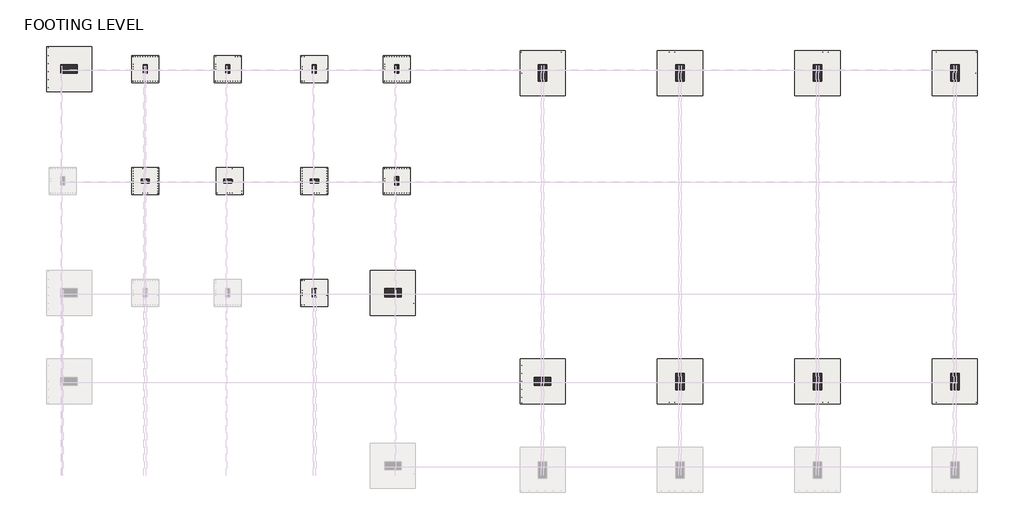
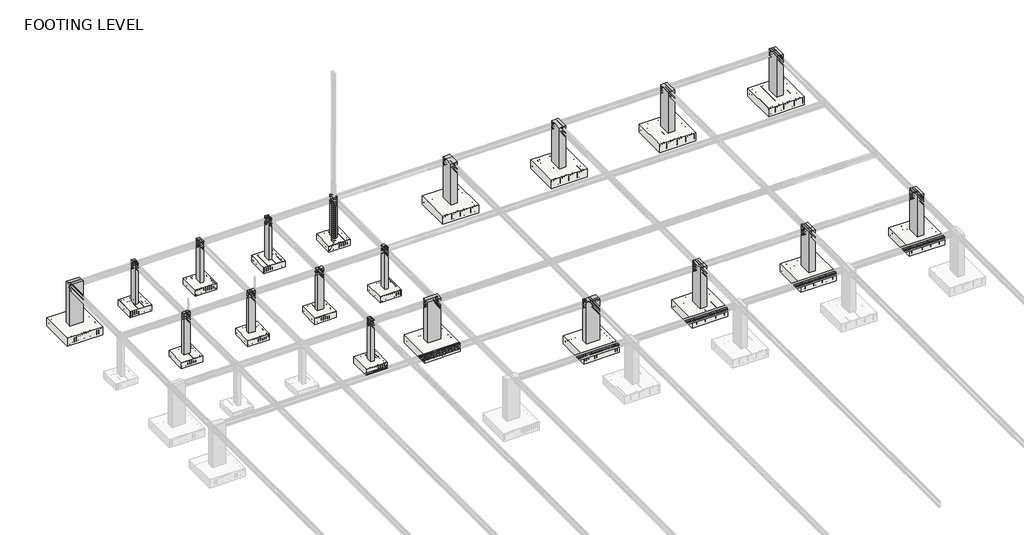
# One storey, part 2 of 19: 19 columns, 19 slabs.
"""IFC4 building model written with IfcOpenShell, lengths in millimetres."""

from ifc_helpers import new_model, si_unit, frame, origin, place, context, project, spatial, polyline, outline, extrude, faceted_brep, transform, mapped, element, save
from components import m_footing_rectangular_2500_x_2500_x_600_5d9c2050

model = new_model("IFC4")

# Units and contexts
model_context = context("Model", 3, world=origin())
ifc_project = project(units=[si_unit("LENGTHUNIT", "METRE", prefix="MILLI")], contexts=[model_context])

# Site, building, storey
site = spatial("IfcSite", under=ifc_project)
building = spatial("IfcBuilding", under=site)
storey = spatial("IfcBuildingStorey", under=building, Name="FOOTING LEVEL", Elevation=-3048.0)

# Columns
placement = place(None, origin())
element("IfcColumn", 1, ObjectType="M_Concrete-Rectangular-Column : 18\" X 36\"", at=placement, inside=storey, context=model_context, shape_type="Brep", body=[
    faceted_brep([(689.5587563, 6154.1794445, -3048.0), (1603.9587563, 6154.1794445, -3048.0), (1603.9587563, 5696.9794445, -3048.0), (689.5587563, 5696.9794445, -3048.0), (689.5587563, 6154.1794445, 0.0), (1603.9587563, 6154.1794445, 0.0), (1603.9587563, 5696.9794445, 0.0), (689.5587563, 5696.9794445, 0.0), (689.5587563, 5811.2794445, 0.0), (689.5587563, 6039.8794445, 0.0)], [[[0, 1, 2, 3]], [[4, 5, 1, 0]], [[5, 6, 2, 1]], [[6, 7, 3, 2]], [[7, 8, 9, 4, 0, 3]], [[4, 9, 8, 7, 6, 5]]]),
])
element("IfcColumn", 2, ObjectType="M_Concrete-Rectangular-Column : 18\" X 36\"", at=placement, inside=storey, context=model_context, shape_type="Brep", body=[
    faceted_brep([(32083.9587563, 553.4794445, -3048.0), (32083.9587563, 1467.8794445, -3048.0), (32541.1587563, 1467.8794445, -3048.0), (32541.1587563, 553.4794445, -3048.0), (32083.9587563, 553.4794445, 0.0), (32083.9587563, 1467.8794445, 0.0), (32198.2587563, 1467.8794445, 0.0), (32426.8587563, 1467.8794445, 0.0), (32541.1587563, 1467.8794445, 0.0), (32541.1587563, 553.4794445, 0.0), (32426.8587563, 553.4794445, 0.0), (32198.2587563, 553.4794445, 0.0)], [[[0, 1, 2, 3]], [[4, 5, 1, 0]], [[5, 6, 7, 8, 2, 1]], [[8, 9, 3, 2]], [[9, 10, 11, 4, 0, 3]], [[4, 11, 10, 9, 8, 7, 6, 5]]]),
])
element("IfcColumn", 3, ObjectType="M_Concrete-Rectangular-Column : 18\" X 36\"", at=placement, inside=storey, context=model_context, shape_type="Brep", body=[
    faceted_brep([(24463.9587563, 553.4794445, -3048.0), (24463.9587563, 1467.8794445, -3048.0), (24921.1587563, 1467.8794445, -3048.0), (24921.1587563, 553.4794445, -3048.0), (24463.9587563, 553.4794445, 0.0), (24463.9587563, 896.3794445, 0.0), (24463.9587563, 1124.9794445, 0.0), (24463.9587563, 1467.8794445, 0.0), (24578.2587563, 1467.8794445, 0.0), (24806.8587563, 1467.8794445, 0.0), (24921.1587563, 1467.8794445, 0.0), (24921.1587563, 1124.9794445, 0.0), (24921.1587563, 896.3794445, 0.0), (24921.1587563, 553.4794445, 0.0), (24806.8587563, 553.4794445, 0.0), (24578.2587563, 553.4794445, 0.0)], [[[0, 1, 2, 3]], [[4, 5, 6, 7, 1, 0]], [[7, 8, 9, 10, 2, 1]], [[10, 11, 12, 13, 3, 2]], [[13, 14, 15, 4, 0, 3]], [[4, 15, 14, 13, 12, 11, 10, 9, 8, 7, 6, 5]]]),
])
element("IfcColumn", 4, ObjectType="M_Concrete-Rectangular-Column : 18\" X 36\"", at=placement, inside=storey, context=model_context, shape_type="Brep", body=[
    faceted_brep([(16843.9587563, 553.4794445, -3048.0), (16843.9587563, 1467.8794445, -3048.0), (17301.1587563, 1467.8794445, -3048.0), (17301.1587563, 553.4794445, -3048.0), (16843.9587563, 553.4794445, 0.0), (16843.9587563, 896.3794445, 0.0), (16843.9587563, 1124.9794445, 0.0), (16843.9587563, 1467.8794445, 0.0), (16958.2587563, 1467.8794445, 0.0), (17186.8587563, 1467.8794445, 0.0), (17301.1587563, 1467.8794445, 0.0), (17301.1587563, 1124.9794445, 0.0), (17301.1587563, 896.3794445, 0.0), (17301.1587563, 553.4794445, 0.0), (17186.8587563, 553.4794445, 0.0), (16958.2587563, 553.4794445, 0.0)], [[[0, 1, 2, 3]], [[4, 5, 6, 7, 1, 0]], [[7, 8, 9, 10, 2, 1]], [[10, 11, 12, 13, 3, 2]], [[13, 14, 15, 4, 0, 3]], [[4, 15, 14, 13, 12, 11, 10, 9, 8, 7, 6, 5]]]),
])
element("IfcColumn", 5, ObjectType="M_Concrete-Rectangular-Column : 18\" X 36\"", at=placement, inside=storey, context=model_context, shape_type="Brep", body=[
    faceted_brep([(9909.7587563, 782.0794445, -3048.0), (8995.3587563, 782.0794445, -3048.0), (8995.3587563, 1239.2794445, -3048.0), (9909.7587563, 1239.2794445, -3048.0), (9909.7587563, 782.0794445, 0.0), (8995.3587563, 782.0794445, 0.0), (8995.3587563, 896.3794445, 0.0), (8995.3587563, 1124.9794445, 0.0), (8995.3587563, 1239.2794445, 0.0), (9909.7587563, 1239.2794445, 0.0), (9909.7587563, 1124.9794445, 0.0), (9909.7587563, 896.3794445, 0.0)], [[[0, 1, 2, 3]], [[4, 5, 1, 0]], [[5, 6, 7, 8, 2, 1]], [[8, 9, 3, 2]], [[9, 10, 11, 4, 0, 3]], [[4, 11, 10, 9, 8, 7, 6, 5]]]),
])
element("IfcColumn", 6, ObjectType="M_Concrete-Rectangular-Column : 18\" X 36\"", at=placement, inside=storey, context=model_context, shape_type="Brep", body=[
    faceted_brep([(9681.1587563, 18574.7794445, -3048.0), (9681.1587563, 17660.3794445, -3048.0), (9223.9587563, 17660.3794445, -3048.0), (9223.9587563, 18574.7794445, -3048.0), (9681.1587563, 18574.7794445, 0.0), (9681.1587563, 18460.4794445, 0.0), (9681.1587563, 18231.8794445, 0.0), (9681.1587563, 17660.3794445, 0.0), (9223.9587563, 17660.3794445, 0.0), (9223.9587563, 18231.8794445, 0.0), (9223.9587563, 18460.4794445, 0.0), (9223.9587563, 18574.7794445, 0.0)], [[[0, 1, 2, 3]], [[4, 5, 6, 7, 1, 0]], [[7, 8, 2, 1]], [[8, 9, 10, 11, 3, 2]], [[11, 4, 0, 3]], [[4, 11, 10, 9, 8, 7, 6, 5]]]),
])
element("IfcColumn", 7, ObjectType="M_Concrete-Rectangular-Column : 18\" X 36\"", at=placement, inside=storey, context=model_context, shape_type="Brep", body=[
    faceted_brep([(17301.1587563, 18574.7794445, -3048.0), (17301.1587563, 17660.3794445, -3048.0), (16843.9587563, 17660.3794445, -3048.0), (16843.9587563, 18574.7794445, -3048.0), (17301.1587563, 18574.7794445, 0.0), (17301.1587563, 18460.4794445, 0.0), (17301.1587563, 18231.8794445, 0.0), (17301.1587563, 17660.3794445, 0.0), (16843.9587563, 17660.3794445, 0.0), (16843.9587563, 18231.8794445, 0.0), (16843.9587563, 18460.4794445, 0.0), (16843.9587563, 18574.7794445, 0.0)], [[[0, 1, 2, 3]], [[4, 5, 6, 7, 1, 0]], [[7, 8, 2, 1]], [[8, 9, 10, 11, 3, 2]], [[11, 4, 0, 3]], [[4, 11, 10, 9, 8, 7, 6, 5]]]),
])
element("IfcColumn", 8, ObjectType="M_Concrete-Rectangular-Column : 18\" X 36\"", at=placement, inside=storey, context=model_context, shape_type="Brep", body=[
    faceted_brep([(24921.1587563, 18574.7794445, -3048.0), (24921.1587563, 17660.3794445, -3048.0), (24463.9587563, 17660.3794445, -3048.0), (24463.9587563, 18574.7794445, -3048.0), (24921.1587563, 18574.7794445, 0.0), (24921.1587563, 18460.4794445, 0.0), (24921.1587563, 18231.8794445, 0.0), (24921.1587563, 17660.3794445, 0.0), (24463.9587563, 17660.3794445, 0.0), (24463.9587563, 18231.8794445, 0.0), (24463.9587563, 18460.4794445, 0.0), (24463.9587563, 18574.7794445, 0.0)], [[[0, 1, 2, 3]], [[4, 5, 6, 7, 1, 0]], [[7, 8, 2, 1]], [[8, 9, 10, 11, 3, 2]], [[11, 4, 0, 3]], [[4, 11, 10, 9, 8, 7, 6, 5]]]),
])
element("IfcColumn", 9, ObjectType="M_Concrete-Rectangular-Column : 18\" X 36\"", at=placement, inside=storey, context=model_context, shape_type="SweptSolid", body=[
    extrude(outline(polyline([(32541.1587563, 18574.7794445), (32541.1587563, 17660.3794445), (32083.9587563, 17660.3794445), (32083.9587563, 18574.7794445), (32541.1587563, 18574.7794445)])), frame((0.0, 0.0, -3048.0), z_axis=(0.0, 0.0, 1.0), x_axis=(1.0, 0.0, 0.0)), (0.0, 0.0, 1.0), 3048.0),
])
element("IfcColumn", 10, ObjectType="M_Concrete-Rectangular-Column : 18\" X 36\"", at=placement, inside=storey, context=model_context, shape_type="SweptSolid", body=[
    extrude(outline(polyline([(-17255.5412437, 18574.7794445), (-16341.1412437, 18574.7794445), (-16341.1412437, 18117.5794445), (-17255.5412437, 18117.5794445), (-17255.5412437, 18574.7794445)])), frame((0.0, 0.0, -3048.0), z_axis=(0.0, 0.0, 1.0), x_axis=(1.0, 0.0, 0.0)), (0.0, 0.0, 1.0), 3048.0),
])
element("IfcColumn", 11, ObjectType="M_Concrete-Rectangular-Column : 9\" X18\"", at=placement, inside=storey, context=model_context, shape_type="Brep", body=[
    faceted_brep([(-12797.8412437, 12250.1794445, -3048.0), (-12340.6412437, 12250.1794445, -3048.0), (-12340.6412437, 12021.5794445, -3048.0), (-12797.8412437, 12021.5794445, -3048.0), (-12797.8412437, 12250.1794445, 0.0), (-12683.5412437, 12250.1794445, 0.0), (-12454.9412437, 12250.1794445, 0.0), (-12340.6412437, 12250.1794445, 0.0), (-12340.6412437, 12250.1794445, -457.2), (-12797.8412437, 12250.1794445, -457.2), (-12340.6412437, 12021.5794445, 0.0), (-12340.6412437, 12021.5794445, -457.2), (-12454.9412437, 12021.5794445, 0.0), (-12683.5412437, 12021.5794445, 0.0), (-12797.8412437, 12021.5794445, 0.0), (-12797.8412437, 12021.5794445, -457.2)], [[[0, 1, 2, 3]], [[4, 5, 6, 7, 8, 1, 0, 9]], [[7, 10, 11, 2, 1, 8]], [[10, 12, 13, 14, 15, 3, 2, 11]], [[14, 4, 9, 0, 3, 15]], [[4, 14, 13, 12, 10, 7, 6, 5]]]),
])
element("IfcColumn", 12, ObjectType="M_Concrete-Rectangular-Column : 9\" X18\"", at=placement, inside=storey, context=model_context, shape_type="Brep", body=[
    faceted_brep([(-3310.9412437, 5696.9794445, -3048.0), (-3310.9412437, 6154.1794445, -3048.0), (-3082.3412437, 6154.1794445, -3048.0), (-3082.3412437, 5696.9794445, -3048.0), (-3310.9412437, 5696.9794445, 0.0), (-3310.9412437, 5811.2794445, 0.0), (-3310.9412437, 6039.8794445, 0.0), (-3310.9412437, 6154.1794445, 0.0), (-3082.3412437, 6154.1794445, 0.0), (-3082.3412437, 6039.8794445, 0.0), (-3082.3412437, 5811.2794445, 0.0), (-3082.3412437, 5696.9794445, 0.0)], [[[0, 1, 2, 3]], [[4, 5, 6, 7, 1, 0]], [[7, 8, 2, 1]], [[8, 9, 10, 11, 3, 2]], [[11, 4, 0, 3]], [[4, 11, 10, 9, 8, 7, 6, 5]]]),
])
element("IfcColumn", 13, ObjectType="M_Concrete-Rectangular-Column : 9\" X18\"", at=placement, inside=storey, context=model_context, shape_type="Brep", body=[
    faceted_brep([(-7768.6412437, 12021.5794445, -3048.0), (-8225.8412437, 12021.5794445, -3048.0), (-8225.8412437, 12250.1794445, -3048.0), (-7768.6412437, 12250.1794445, -3048.0), (-7768.6412437, 12021.5794445, 0.0), (-7882.9412437, 12021.5794445, 0.0), (-8111.5412437, 12021.5794445, 0.0), (-8225.8412437, 12021.5794445, 0.0), (-8225.8412437, 12021.5794445, -457.2), (-7768.6412437, 12021.5794445, -457.2), (-8225.8412437, 12250.1794445, 0.0), (-8225.8412437, 12250.1794445, -457.2), (-8111.5412437, 12250.1794445, 0.0), (-7882.9412437, 12250.1794445, 0.0), (-7768.6412437, 12250.1794445, 0.0), (-7768.6412437, 12250.1794445, -457.2)], [[[0, 1, 2, 3]], [[4, 5, 6, 7, 8, 1, 0, 9]], [[7, 10, 11, 2, 1, 8]], [[10, 12, 13, 14, 15, 3, 2, 11]], [[14, 4, 9, 0, 3, 15]], [[4, 14, 13, 12, 10, 7, 6, 5]]]),
])
element("IfcColumn", 14, ObjectType="M_Concrete-Rectangular-Column : 9\" X18\"", at=placement, inside=storey, context=model_context, shape_type="Brep", body=[
    faceted_brep([(-2968.0412437, 12021.5794445, -3048.0), (-3425.2412437, 12021.5794445, -3048.0), (-3425.2412437, 12250.1794445, -3048.0), (-2968.0412437, 12250.1794445, -3048.0), (-2968.0412437, 12021.5794445, 0.0), (-3082.3412437, 12021.5794445, 0.0), (-3310.9412437, 12021.5794445, 0.0), (-3425.2412437, 12021.5794445, 0.0), (-3425.2412437, 12021.5794445, -457.2), (-2968.0412437, 12021.5794445, -457.2), (-3425.2412437, 12250.1794445, 0.0), (-3425.2412437, 12250.1794445, -457.2), (-3310.9412437, 12250.1794445, 0.0), (-3082.3412437, 12250.1794445, 0.0), (-2968.0412437, 12250.1794445, 0.0), (-2968.0412437, 12250.1794445, -457.2)], [[[0, 1, 2, 3]], [[4, 5, 6, 7, 8, 1, 0, 9]], [[7, 10, 11, 2, 1, 8]], [[10, 12, 13, 14, 15, 3, 2, 11]], [[14, 4, 9, 0, 3, 15]], [[4, 14, 13, 12, 10, 7, 6, 5]]]),
])
element("IfcColumn", 15, ObjectType="M_Concrete-Rectangular-Column : 9\" X18\"", at=placement, inside=storey, context=model_context, shape_type="Brep", body=[
    faceted_brep([(1489.6587563, 12364.4794445, -3048.0), (1489.6587563, 11907.2794445, -3048.0), (1261.0587563, 11907.2794445, -3048.0), (1261.0587563, 12364.4794445, -3048.0), (1489.6587563, 12364.4794445, 0.0), (1489.6587563, 11907.2794445, 0.0), (1489.6587563, 11907.2794445, -457.2), (1489.6587563, 12364.4794445, -457.2), (1261.0587563, 11907.2794445, 0.0), (1261.0587563, 11907.2794445, -457.2), (1261.0587563, 12021.5794445, 0.0), (1261.0587563, 12250.1794445, 0.0), (1261.0587563, 12364.4794445, 0.0), (1261.0587563, 12364.4794445, -457.2)], [[[0, 1, 2, 3]], [[4, 5, 6, 1, 0, 7]], [[5, 8, 9, 2, 1, 6]], [[8, 10, 11, 12, 13, 3, 2, 9]], [[12, 4, 7, 0, 3, 13]], [[4, 12, 11, 10, 8, 5]]]),
])
element("IfcColumn", 16, ObjectType="M_Concrete-Rectangular-Column : 9\" X18\"", at=placement, inside=storey, context=model_context, shape_type="Brep", body=[
    faceted_brep([(-7882.9412437, 18574.7794445, -3048.0), (-7882.9412437, 18117.5794445, -3048.0), (-8111.5412437, 18117.5794445, -3048.0), (-8111.5412437, 18574.7794445, -3048.0), (-7882.9412437, 18574.7794445, 0.0), (-7882.9412437, 18460.4794445, 0.0), (-7882.9412437, 18231.8794445, 0.0), (-7882.9412437, 18117.5794445, 0.0), (-8111.5412437, 18117.5794445, 0.0), (-8111.5412437, 18231.8794445, 0.0), (-8111.5412437, 18460.4794445, 0.0), (-8111.5412437, 18574.7794445, 0.0)], [[[0, 1, 2, 3]], [[4, 5, 6, 7, 1, 0]], [[7, 8, 2, 1]], [[8, 9, 10, 11, 3, 2]], [[11, 4, 0, 3]], [[4, 11, 10, 9, 8, 7, 6, 5]]]),
])
element("IfcColumn", 17, ObjectType="M_Concrete-Rectangular-Column : 9\" X18\"", at=placement, inside=storey, context=model_context, shape_type="Brep", body=[
    faceted_brep([(-12454.9412437, 18574.7794445, -3048.0), (-12454.9412437, 18117.5794445, -3048.0), (-12683.5412437, 18117.5794445, -3048.0), (-12683.5412437, 18574.7794445, -3048.0), (-12454.9412437, 18574.7794445, 0.0), (-12454.9412437, 18460.4794445, 0.0), (-12454.9412437, 18231.8794445, 0.0), (-12454.9412437, 18117.5794445, 0.0), (-12683.5412437, 18117.5794445, 0.0), (-12683.5412437, 18231.8794445, 0.0), (-12683.5412437, 18460.4794445, 0.0), (-12683.5412437, 18574.7794445, 0.0)], [[[0, 1, 2, 3]], [[4, 5, 6, 7, 1, 0]], [[7, 8, 2, 1]], [[8, 9, 10, 11, 3, 2]], [[11, 4, 0, 3]], [[4, 11, 10, 9, 8, 7, 6, 5]]]),
])
element("IfcColumn", 18, ObjectType="M_Concrete-Rectangular-Column : 9\" X18\"", at=placement, inside=storey, context=model_context, shape_type="Brep", body=[
    faceted_brep([(-3082.3412437, 18574.7794445, -3048.0), (-3082.3412437, 18117.5794445, -3048.0), (-3310.9412437, 18117.5794445, -3048.0), (-3310.9412437, 18574.7794445, -3048.0), (-3082.3412437, 18574.7794445, 0.0), (-3082.3412437, 18460.4794445, 0.0), (-3082.3412437, 18231.8794445, 0.0), (-3082.3412437, 18117.5794445, 0.0), (-3310.9412437, 18117.5794445, 0.0), (-3310.9412437, 18231.8794445, 0.0), (-3310.9412437, 18460.4794445, 0.0), (-3310.9412437, 18574.7794445, 0.0)], [[[0, 1, 2, 3]], [[4, 5, 6, 7, 1, 0]], [[7, 8, 2, 1]], [[8, 9, 10, 11, 3, 2]], [[11, 4, 0, 3]], [[4, 11, 10, 9, 8, 7, 6, 5]]]),
])
element("IfcColumn", 19, ObjectType="M_Concrete-Rectangular-Column : 9\" X18\"", at=placement, inside=storey, context=model_context, shape_type="SweptSolid", body=[
    extrude(outline(polyline([(1489.6587563, 18574.7794445), (1489.6587563, 18117.5794445), (1261.0587563, 18117.5794445), (1261.0587563, 18574.7794445), (1489.6587563, 18574.7794445)])), frame((0.0, 0.0, -3048.0), z_axis=(0.0, 0.0, 1.0), x_axis=(1.0, 0.0, 0.0)), (0.0, 0.0, 1.0), 3048.0),
])

# Slabs
element("IfcSlab", 20, ObjectType="M_Footing-Rectangular : 1500 X1500 X450", at=placement, inside=storey, context=model_context, shape_type="SweptSolid", body=[
    extrude(outline(polyline([(-2446.6412437, 6675.5794445), (-2446.6412437, 5175.5794445), (-3946.6412437, 5175.5794445), (-3946.6412437, 6675.5794445), (-2446.6412437, 6675.5794445)])), frame((0.0, 0.0, -3498.0), z_axis=(0.0, 0.0, 1.0), x_axis=(1.0, 0.0, 0.0)), (0.0, 0.0, 1.0), 450.0),
])
element("IfcSlab", 21, ObjectType="M_Footing-Rectangular : 1500 X1500 X450", at=placement, inside=storey, context=model_context, shape_type="SweptSolid", body=[
    extrude(outline(polyline([(-11819.2412437, 12885.8794445), (-11819.2412437, 11385.8794445), (-13319.2412437, 11385.8794445), (-13319.2412437, 12885.8794445), (-11819.2412437, 12885.8794445)])), frame((0.0, 0.0, -3498.0), z_axis=(0.0, 0.0, 1.0), x_axis=(1.0, 0.0, 0.0)), (0.0, 0.0, 1.0), 450.0),
])
element("IfcSlab", 22, ObjectType="M_Footing-Rectangular : 1500 X1500 X450", at=placement, inside=storey, context=model_context, shape_type="SweptSolid", body=[
    extrude(outline(polyline([(-7147.2412437, 12885.8794445), (-7147.2412437, 11385.8794445), (-8647.2412437, 11385.8794445), (-8647.2412437, 12885.8794445), (-7147.2412437, 12885.8794445)])), frame((0.0, 0.0, -3498.0), z_axis=(0.0, 0.0, 1.0), x_axis=(1.0, 0.0, 0.0)), (0.0, 0.0, 1.0), 450.0),
])
element("IfcSlab", 23, ObjectType="M_Footing-Rectangular : 1500 X1500 X450", at=placement, inside=storey, context=model_context, shape_type="SweptSolid", body=[
    extrude(outline(polyline([(-2446.6412437, 12885.8794445), (-2446.6412437, 11385.8794445), (-3946.6412437, 11385.8794445), (-3946.6412437, 12885.8794445), (-2446.6412437, 12885.8794445)])), frame((0.0, 0.0, -3498.0), z_axis=(0.0, 0.0, 1.0), x_axis=(1.0, 0.0, 0.0)), (0.0, 0.0, 1.0), 450.0),
])
element("IfcSlab", 24, ObjectType="M_Footing-Rectangular : 1500 X1500 X450", at=placement, inside=storey, context=model_context, shape_type="SweptSolid", body=[
    extrude(outline(polyline([(2125.3587563, 12885.8794445), (2125.3587563, 11385.8794445), (625.3587563, 11385.8794445), (625.3587563, 12885.8794445), (2125.3587563, 12885.8794445)])), frame((0.0, 0.0, -3498.0), z_axis=(0.0, 0.0, 1.0), x_axis=(1.0, 0.0, 0.0)), (0.0, 0.0, 1.0), 450.0),
])
element("IfcSlab", 25, ObjectType="M_Footing-Rectangular : 1500 X1500 X450", at=placement, inside=storey, context=model_context, shape_type="SweptSolid", body=[
    extrude(outline(polyline([(2125.3587563, 19096.1794445), (2125.3587563, 17596.1794445), (625.3587563, 17596.1794445), (625.3587563, 19096.1794445), (2125.3587563, 19096.1794445)])), frame((0.0, 0.0, -3498.0), z_axis=(0.0, 0.0, 1.0), x_axis=(1.0, 0.0, 0.0)), (0.0, 0.0, 1.0), 450.0),
])
element("IfcSlab", 26, ObjectType="M_Footing-Rectangular : 1500 X1500 X450", at=placement, inside=storey, context=model_context, shape_type="SweptSolid", body=[
    extrude(outline(polyline([(-2446.6412437, 19096.1794445), (-2446.6412437, 17596.1794445), (-3946.6412437, 17596.1794445), (-3946.6412437, 19096.1794445), (-2446.6412437, 19096.1794445)])), frame((0.0, 0.0, -3498.0), z_axis=(0.0, 0.0, 1.0), x_axis=(1.0, 0.0, 0.0)), (0.0, 0.0, 1.0), 450.0),
])
element("IfcSlab", 27, ObjectType="M_Footing-Rectangular : 1500 X1500 X450", at=placement, inside=storey, context=model_context, shape_type="SweptSolid", body=[
    extrude(outline(polyline([(-7247.2412437, 19096.1794445), (-7247.2412437, 17596.1794445), (-8747.2412437, 17596.1794445), (-8747.2412437, 19096.1794445), (-7247.2412437, 19096.1794445)])), frame((0.0, 0.0, -3498.0), z_axis=(0.0, 0.0, 1.0), x_axis=(1.0, 0.0, 0.0)), (0.0, 0.0, 1.0), 450.0),
])
element("IfcSlab", 28, ObjectType="M_Footing-Rectangular : 1500 X1500 X450", at=placement, inside=storey, context=model_context, shape_type="SweptSolid", body=[
    extrude(outline(polyline([(-11819.2412437, 19096.1794445), (-11819.2412437, 17596.1794445), (-13319.2412437, 17596.1794445), (-13319.2412437, 19096.1794445), (-11819.2412437, 19096.1794445)])), frame((0.0, 0.0, -3498.0), z_axis=(0.0, 0.0, 1.0), x_axis=(1.0, 0.0, 0.0)), (0.0, 0.0, 1.0), 450.0),
])
element("IfcSlab", 29, ObjectType="M_Footing-Rectangular : 2500 X 2500 X 600", at=placement, inside=storey, context=model_context, shape_type="SweptSolid", body=[
    extrude(outline(polyline([(2396.7587563, 7175.5794445), (2396.7587563, 4675.5794445), (-103.2412437, 4675.5794445), (-103.2412437, 7175.5794445), (2396.7587563, 7175.5794445)])), frame((0.0, 0.0, -3648.0), z_axis=(0.0, 0.0, 1.0), x_axis=(1.0, 0.0, 0.0)), (0.0, 0.0, 1.0), 600.0),
])
element("IfcSlab", 30, ObjectType="M_Footing-Rectangular : 2500 X 2500 X 600", at=placement, inside=storey, context=model_context, shape_type="SweptSolid", body=[
    extrude(outline(polyline([(-15548.3412437, 19596.1794445), (-15548.3412437, 17096.1794445), (-18048.3412437, 17096.1794445), (-18048.3412437, 19596.1794445), (-15548.3412437, 19596.1794445)])), frame((0.0, 0.0, -3648.0), z_axis=(0.0, 0.0, 1.0), x_axis=(1.0, 0.0, 0.0)), (0.0, 0.0, 1.0), 600.0),
])
m_footing_rectangular_2500_x_2500_x_600_shape = m_footing_rectangular_2500_x_2500_x_600_5d9c2050(model_context)
element("IfcSlab", 31, ObjectType="M_Footing-Rectangular : 2500 X 2500 X 600", at=placement, inside=storey, context=model_context, shape_type="MappedRepresentation", body=[
    mapped(m_footing_rectangular_2500_x_2500_x_600_shape, transform((32312.5587563, 1010.6794445, -3048.0), x_axis=(1.0, 0.0, 0.0), y_axis=(0.0, 1.0, 0.0), z_axis=(0.0, 0.0, 1.0))),
])
element("IfcSlab", 32, ObjectType="M_Footing-Rectangular : 2500 X 2500 X 600", at=placement, inside=storey, context=model_context, shape_type="MappedRepresentation", body=[
    mapped(m_footing_rectangular_2500_x_2500_x_600_shape, transform((24692.5587563, 1010.6794445, -3048.0), x_axis=(1.0, 0.0, 0.0), y_axis=(0.0, 1.0, 0.0), z_axis=(0.0, 0.0, 1.0))),
])
element("IfcSlab", 33, ObjectType="M_Footing-Rectangular : 2500 X 2500 X 600", at=placement, inside=storey, context=model_context, shape_type="MappedRepresentation", body=[
    mapped(m_footing_rectangular_2500_x_2500_x_600_shape, transform((17072.5587563, 1010.6794445, -3048.0), x_axis=(1.0, 0.0, 0.0), y_axis=(0.0, 1.0, 0.0), z_axis=(0.0, 0.0, 1.0))),
])
element("IfcSlab", 34, ObjectType="M_Footing-Rectangular : 2500 X 2500 X 600", at=placement, inside=storey, context=model_context, shape_type="MappedRepresentation", body=[
    mapped(m_footing_rectangular_2500_x_2500_x_600_shape, transform((9452.5587563, 1010.6794445, -3048.0), x_axis=(1.0, 0.0, 0.0), y_axis=(0.0, 1.0, 0.0), z_axis=(0.0, 0.0, 1.0))),
])
element("IfcSlab", 35, ObjectType="M_Footing-Rectangular : 2500 X 2500 X 600", at=placement, inside=storey, context=model_context, shape_type="MappedRepresentation", body=[
    mapped(m_footing_rectangular_2500_x_2500_x_600_shape, transform((9452.5587563, 18117.5794445, -3048.0), x_axis=(1.0, 0.0, 0.0), y_axis=(0.0, 1.0, 0.0), z_axis=(0.0, 0.0, 1.0))),
])
element("IfcSlab", 36, ObjectType="M_Footing-Rectangular : 2500 X 2500 X 600", at=placement, inside=storey, context=model_context, shape_type="MappedRepresentation", body=[
    mapped(m_footing_rectangular_2500_x_2500_x_600_shape, transform((17072.5587563, 18117.5794445, -3048.0), x_axis=(1.0, 0.0, 0.0), y_axis=(0.0, 1.0, 0.0), z_axis=(0.0, 0.0, 1.0))),
])
element("IfcSlab", 37, ObjectType="M_Footing-Rectangular : 2500 X 2500 X 600", at=placement, inside=storey, context=model_context, shape_type="MappedRepresentation", body=[
    mapped(m_footing_rectangular_2500_x_2500_x_600_shape, transform((24692.5587563, 18117.5794445, -3048.0), x_axis=(1.0, 0.0, 0.0), y_axis=(0.0, 1.0, 0.0), z_axis=(0.0, 0.0, 1.0))),
])
element("IfcSlab", 38, ObjectType="M_Footing-Rectangular : 2500 X 2500 X 600", at=placement, inside=storey, context=model_context, shape_type="MappedRepresentation", body=[
    mapped(m_footing_rectangular_2500_x_2500_x_600_shape, transform((32312.5587563, 18117.5794445, -3048.0), x_axis=(1.0, 0.0, 0.0), y_axis=(0.0, 1.0, 0.0), z_axis=(0.0, 0.0, 1.0))),
])

save(model, "model.ifc")

# Revit data of these elements
# Type "M_Concrete-Rectangular-Column : 18\" X 36\""
#   b = 457.2 mm
#   h = 914.4 mm
#   Structural Material [instance default] = Concrete, Cast-in-Place gray
# Type "M_Concrete-Rectangular-Column : 9\" X18\""
#   b = 228.6 mm
#   h = 457.2 mm
#   Structural Material [instance default] = Concrete, Cast-in-Place gray
# Type "M_Footing-Rectangular : 1500 X1500 X450"
#   Width = 1500 mm
#   Length = 1500 mm
#   Foundation Thickness = 450 mm
#   Structural Material [instance default] = Concrete, Cast-in-Place gray
#   Assembly Code = ""
# Type "M_Footing-Rectangular : 2500 X 2500 X 600"
#   Width = 2500 mm
#   Length = 2500 mm
#   Foundation Thickness = 600 mm
#   Structural Material [instance default] = Concrete, Cast-in-Place gray
#   Assembly Code = ""
# Elements 1, 2, 3, 4, 5, 6, 7, 8, 9, 10 (IfcColumn, "M_Concrete-Rectangular-Column : 18\" X 36\"")
#   Structural Material = Concrete, Cast-in-Place gray
#   Phase Created = New Construction
#   Materials on its faces: "Concrete, Cast-in-Place gray"
# Elements 11, 12, 13, 14, 15, 16, 17, 18, 19 (IfcColumn, "M_Concrete-Rectangular-Column : 9\" X18\"")
#   Structural Material = Concrete, Cast-in-Place gray
#   Phase Created = New Construction
#   Materials on its faces: "Concrete, Cast-in-Place gray"
# Elements 20, 21, 22, 23, 24, 25, 26, 27, 28 (IfcSlab, "M_Footing-Rectangular : 1500 X1500 X450")
#   Structural Material = Concrete, Cast-in-Place gray
#   Phase Created = New Construction
#   Materials on its faces: "Concrete, Cast-in-Place gray"
# Elements 29, 30, 31, 32, 33, 34, 35, 36, 37, 38 (IfcSlab, "M_Footing-Rectangular : 2500 X 2500 X 600")
#   Structural Material = Concrete, Cast-in-Place gray
#   Phase Created = New Construction
#   Materials on its faces: "Concrete, Cast-in-Place gray"
# Materials
#   "Concrete, Cast-in-Place gray": class "Concrete", colour RGB 192 192 192, transparency 0, Description = "Cast-in-place concrete", Cost = 0
